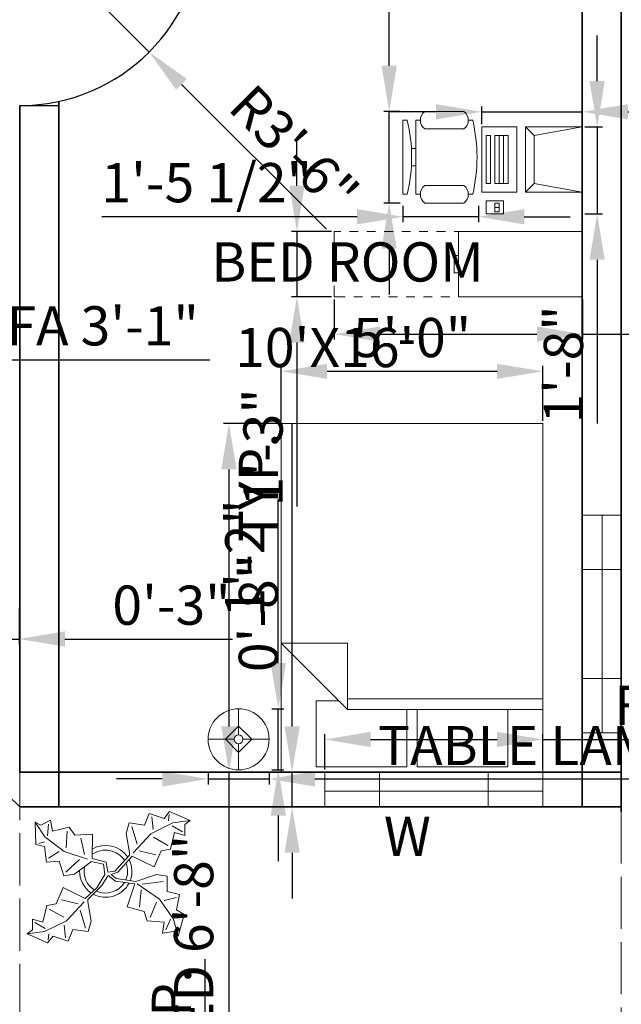
# Model space of a CAD drawing. Units: inches. Extents: x 1956 to 4770, y 1551 to 2596.
# Tile 4 of 10: x 2363 to 2501, y 1865 to 2091. Entities that reach past the tile are written whole.
import ezdxf

# ---------------------------------------------------------------- set-up
doc = ezdxf.new("R2010")
doc.units = ezdxf.units.IN
doc.linetypes.add('ACAD_ISO02W100', pattern=[15, 12, -3])
for name, color, linetype, lineweight in [('A-ANNO-DIMS', 2, 'Continuous', 18), ('A-ANNO-TEXT', 7, 'Continuous', 18), ('A-AREA-IDEN', 7, 'Continuous', 18), ('A-DOOR', 3, 'Continuous', 25), ('A-EQPM', 9, 'Continuous', 18), ('A-FLOR-OVHD', 8, 'ACAD_ISO02W100', 18), ('A-FURN', 8, 'Continuous', 18), ('A-GLAZ', 4, 'Continuous', 18), ('A-WALL', 7, 'Continuous', 35), ('L-PLNT', 116, 'Continuous', 18)]:
    doc.layers.add(name, color=color, linetype=linetype, lineweight=lineweight)
doc.styles.get("Standard").update_dxf_attribs({"font": 'arial.ttf'})
doc.dimstyles.new('ISO-25', dxfattribs={"dimtxt": 9, "dimasz": 10.5, "dimexe": 1.25, "dimexo": 0.625, "dimgap": 2, "dimtad": 1, "dimdec": 1, "dimlunit": 4, "dimtxsty": 'Standard', "dimcen": 2.5, "dimadec": 0, "dimazin": 0, "dimtfac": 1, "dimtdec": 1, "dimtmove": 0, "dimatfit": 3, "dimfxl": 1, "dimarcsym": 0})

# ---------------------------------------------------------------- blocks, each defined once
blk = doc.blocks.new('*D1')
at = {"layer": 'A-ANNO-DIMS', "color": 0, "lineweight": -2, "transparency": 16777216}
for p, q in [((2501.88, 2309.09), (2599.11, 2309.09)), ((2597.86, 2298.59), (2597.86, 1767.59)), ((2501.88, 1757.09), (2599.11, 1757.09))]:
    blk.add_line(p, q, dxfattribs=at)
at = {"layer": 'A-ANNO-DIMS', "color": 0, "transparency": 16777216}
for points in [[(2596.11, 2298.59), (2599.61, 2298.59), (2597.86, 2309.09)], [(2596.11, 1767.59), (2599.61, 1767.59), (2597.86, 1757.09)]]:
    blk.add_solid(points, dxfattribs=at)
at = {"layer": 'Defpoints', "color": 0, "transparency": 16777216}
for p in [(2501.25, 2309.09), (2501.25, 1757.09), (2597.86, 1757.09)]:
    blk.add_point(p, dxfattribs=at)
at = {"layer": 'A-ANNO-DIMS', "color": 0, "transparency": 16777216, "insert": (2591.27, 2033.09), "char_height": 9, "attachment_point": 5, "rotation": 90}
blk.add_mtext("46'", dxfattribs=at)
blk = doc.blocks.new('Bed - Queen')
for p, q in [((0, -80.00003), (0, 0)), ((0, 0), (59.99999, 0)), ((59.99999, 0), (59.99999, -80.00003)), ((7.99999, -1.2), (28.79998, -1.2)), ((7.99999, -14.4), (7.99999, -1.2)), ((28.79998, -1.2), (28.79998, -14.4)), ((31.19999, -1.2), (51.99999, -1.2)), ((31.19999, -14.4), (31.19999, -1.2)), ((51.99999, -1.2), (51.99999, -16.4)), ((0, -14.4), (44.8, -14.4)), ((59.99999, -29.6), (44.8, -14.4)), ((44.8, -14.4), (44.8, -29.6)), ((44.8, -16.8), (0, -16.8)), ((51.99999, -16.4), (46.79936, -16.4)), ((44.8, -29.6), (59.99999, -29.6)), ((59.99999, -80.00003), (0, -80.00003))]:
    blk.add_line(p, q)
blk = doc.blocks.new('Lamp - Table')
for p, q in [((0, 7), (0, 1)), ((0, 3), (-3, 0)), ((3, 0), (0, 3)), ((-1, 0), (-7, 0)), ((-3, 0), (0, -3)), ((0, -3), (3, 0)), ((1, 0), (7, 0)), ((0, -1), (0, -7))]:
    blk.add_line(p, q)
for radius in [7, 1]:
    blk.add_circle((0, 0), radius)
blk = doc.blocks.new('Computer Terminal')
for p, q in [((-10, 11.5), (5, 11.5)), ((-8, 0.5), (-10, 11.5)), ((-10, -1.5), (-10, 11.5)), ((5, 11.5), (3, 0.5)), ((5, 11.5), (5, -1.5)), ((-10, -1.5), (-8, 0.5)), ((3, 0.5), (-8, 0.5)), ((3, 0.5), (5, -1.5)), ((5, -1.5), (-10, -1.5)), ((-10, -11.5), (-10, -3.5)), ((-10, -3.5), (5, -3.5)), ((5, -3.5), (5, -11.5)), ((-8, -5.5), (-8, -8.5)), ((3, -5.5), (-8, -5.5)), ((3, -6.5), (-8, -6.5)), ((3, -8.5), (3, -5.5)), ((10, -6.5), (7, -6.5)), ((7, -6.5), (7, -10.5)), ((10, -10.5), (10, -6.5)), ((-8, -7.5), (3, -7.5)), ((-8, -8.5), (3, -8.5)), ((9.5, -7.5), (7.5, -7.5)), ((7.5, -7.5), (7.5, -8.5)), ((7.5, -8.5), (9.5, -8.5)), ((8.5, -7.5), (8.5, -8.5)), ((9.5, -8.5), (9.5, -7.5)), ((-8, -9.5), (-8, -10.5)), ((3, -9.5), (-8, -9.5)), ((-8, -10.5), (3, -10.5)), ((3, -10.5), (3, -9.5)), ((7, -10.5), (10, -10.5)), ((5, -11.5), (-10, -11.5))]:
    blk.add_line(p, q)
blk = doc.blocks.new('File Cabinet - Letter')
for p, q in [((0, 0), (15, 0)), ((0, -28.5), (0, 0)), ((15, 0), (15, -28.5)), ((15, -28.5), (0, -28.5)), ((0, -29.5), (0, -28.5)), ((5.5, -28.5), (5.5, -29.5)), ((9.5, -29.5), (9.5, -28.5)), ((0, -33.5), (0, -31.5)), ((5.5, -29.5), (9.5, -29.5)), ((15, -30.5), (15, -32.5)), ((0, -37.5), (0, -35.5)), ((15, -34.5), (15, -36.5)), ((0, -41.5), (0, -39.5)), ((15, -38.5), (15, -40.5)), ((15, -42.5), (15, -44.5)), ((0, -45.5), (0, -43.5)), ((15, -46.5), (15, -48.5)), ((0, -49.5), (0, -47.5)), ((0, -53.5), (0, -51.5)), ((15, -50.5), (15, -52.5)), ((0, -57), (0, -55.5)), ((15, -54.5), (15, -57)), ((2.5, -57), (0, -57)), ((6.5, -57), (4.5, -57)), ((10.5, -57), (8.5, -57)), ((15, -57), (12.5, -57))]:
    blk.add_line(p, q)
blk = doc.blocks.new('Chair - Desk')
for p, q in [((-8.5, 0), (-8.5, -1)), ((-8.5, 0), (8.5, 0)), ((8.5, 0), (8.5, -1)), ((-2, -3), (-2, -1.9355)), ((2, -1.9576), (2, -3)), ((-8.5, -3), (-8.5, -4)), ((-8.5, -3), (8.5, -3)), ((8.5, -3), (8.5, -4)), ((-10.5, -5), (-10.5, -14)), ((-6.5, -14), (-6.5, -5)), ((6.5, -5), (6.5, -14)), ((10.5, -14), (10.5, -5)), ((-8.5, -15), (-8.5, -16)), ((8.5, -15), (8.5, -16))]:
    blk.add_line(p, q)
for centre, radius, start, end in [((0, 34.625), 36.625, 256.5803, 283.4197), ((-8.5, -6.5), 2.5, 36.8699, 143.1301), ((8.5, -6.5), 2.5, 36.8699, 143.1301), ((-8.5, -12.5), 2.5, 216.8699, 323.1301), ((8.5, -12.5), 2.5, 216.8699, 323.1301), ((0, 19.625), 36.625, 256.5803, 283.4197)]:
    blk.add_arc(centre, radius, start, end)
blk = doc.blocks.new('Plant - Rubber or Philodendron')
for p, q in [((13.3837, 12.301), (14.68, 13.9039)), ((14.68, 13.9039), (19.3848, 11.8146)), ((-16.2005, 11.4774), (-13.9899, 8.1064)), ((-16.2005, 11.4774), (-14.8639, 10.7964)), ((-16.0159, 6.3329), (-16.2005, 11.4774)), ((-14.8639, 10.7964), (-12.6195, 11.8975)), ((-12.6195, 11.8975), (-12.1909, 9.4345)), ((8.8871, 10.7908), (9.9809, 13.4933)), ((9.9809, 13.4933), (13.3837, 12.301)), ((15.3859, 11.3055), (10.3916, 8.7942)), ((10.5828, 12.6946), (10.8893, 9.7953)), ((14.5816, 13.2037), (14.3848, 11.8033)), ((19.3848, 11.8146), (15.3859, 11.3055)), ((19.3848, 11.8146), (18.1868, 10.9119)), ((-13.3174, 8.325), (-13.0735, 11.0065)), ((-12.1909, 9.4345), (-8.3829, 10.3)), ((-8.8369, 9.409), (-9.0894, 5.6095)), ((-8.3829, 10.3), (-7.0549, 8.501)), ((4.6914, 8.8812), (5.3859, 11.2828)), ((5.3859, 11.2828), (8.8871, 10.7908)), ((5.9878, 10.4842), (7.1971, 6.3869)), ((15.7909, 9.1065), (14.8995, 5.3044)), ((15.2875, 10.6053), (17.5907, 9.2105)), ((18.1925, 8.4119), (15.7909, 9.1065)), ((18.1868, 10.9119), (18.1925, 8.4119)), ((-15.3434, 6.5514), (-13.9984, 6.9884)), ((-13.9899, 8.1064), (-9.5434, 4.7185)), ((-7.0549, 8.501), (-3.0284, 8.6941)), ((-4.8529, 4.012), (-5.7184, 7.82)), ((-3.0284, 8.6941), (-3.0709, 3.1041)), ((4.6914, 8.8812), (5.5014, 4.4831)), ((10.3916, 8.7942), (6.2847, 4.4028)), ((14.2977, 6.1031), (10.9934, 7.9956)), ((-14.0069, 5.8704), (-16.0159, 6.3329)), ((-13.5868, 2.2894), (-14.0069, 5.8704)), ((-13.1329, 3.1804), (-10.6614, 4.727)), ((-9.5434, 4.7185), (-4.1917, 2.9888)), ((7.7005, 4.8881), (11.5025, 3.9967)), ((12.7005, 4.8994), (11.1089, 1.1958)), ((14.8995, 5.3044), (12.7005, 4.8994)), ((-10.6784, 2.491), (-13.5868, 2.2894)), ((-9.5858, -0.8715), (-10.6784, 2.491)), ((-9.1318, 0.0195), (-5.9793, 2.9025)), ((-3.5248, 2.2131), (-3.3011, 2.4355)), ((-3.3011, 2.4355), (-0.5306, 1.7947)), ((-3.0709, 3.1041), (0.0797, 2.3163)), ((0.0797, 2.3163), (0.4866, -0.031)), ((2.1141, 0.2298), (5.4346, 3.9146)), ((6.1032, 3.6844), (2.8262, -0.031)), ((5.4346, 3.9146), (5.5014, 4.4831)), ((11.1089, 1.1958), (6.1032, 3.6844)), ((-7.1228, -0.443), (-3.5248, 2.2131)), ((-0.5306, 1.7947), (-0.2255, -0.5527)), ((-0.5306, 1.7947), (-0.5306, 1.7947)), ((0.4866, -0.031), (2.1141, 0.2298)), ((-7.1228, -0.443), (-9.5858, -0.8715)), ((-2.019, -3.6148), (-0.2255, -0.5527)), ((-0.9375, -3.1608), (0.5883, -0.8135)), ((0.5883, -0.8135), (2.2447, -2.0916)), ((2.8262, -0.031), (1.3003, -0.5527)), ((1.3003, -0.5527), (2.4193, -1.4655)), ((2.2447, -2.0916), (6.7108, -2.6626)), ((2.4193, -1.4655), (6.895, -2.1175)), ((11.6605, -0.5413), (6.895, -2.1175)), ((8.3544, -2.7453), (13.1973, -2.1704)), ((11.6605, -0.5413), (14.1354, -0.8948)), ((14.1354, -0.8948), (14.1354, -4.4304)), ((-11.3237, -7.2629), (-9.7321, -3.5593)), ((-9.7321, -3.5593), (-4.7264, -6.0479)), ((-2.019, -3.6148), (-4.7264, -6.0479)), ((-4.0579, -6.2781), (-0.9375, -3.1608)), ((4.943, -7.9659), (6.7108, -2.6626)), ((12.3677, -6.1981), (7.219, -2.6772)), ((8.125, -4.0768), (7.7715, -7.9659)), ((14.1354, -4.4304), (16.9638, -5.1375)), ((-6.3237, -7.2516), (-10.1257, -6.3602)), ((-4.1246, -6.8466), (-4.0579, -6.2781)), ((15.5496, -10.7943), (12.3677, -6.1981)), ((16.2567, -5.8446), (13.4283, -6.5517)), ((16.9638, -5.1375), (16.2567, -8.673)), ((-14.4141, -11.4699), (-13.5228, -7.6679)), ((-13.5228, -7.6679), (-11.3237, -7.2629)), ((-12.921, -8.4665), (-9.6166, -10.359)), ((-9.0148, -11.1577), (-4.9047, -6.8122)), ((-4.611, -12.8477), (-5.8203, -8.7504)), ((-3.3146, -11.2447), (-4.1246, -6.8466)), ((8.8321, -9.0266), (4.943, -7.9659)), ((9.5392, -11.1479), (8.8321, -9.0266)), ((10.2463, -10.4408), (11.6605, -6.9053)), ((16.2567, -8.673), (18.0245, -9.7337)), ((-16.8157, -10.7754), (-14.4141, -11.4699)), ((-16.8101, -13.2754), (-16.8157, -10.7754)), ((-14.0091, -13.669), (-9.0148, -11.1577)), ((-3.3146, -11.2447), (-4.0092, -13.6463)), ((13.4283, -11.5015), (9.5392, -11.1479)), ((14.8425, -10.7943), (13.7819, -13.2692)), ((16.6103, -14.6834), (15.5496, -10.7943)), ((17.3174, -9.7337), (15.9032, -9.7337)), ((18.0245, -9.7337), (16.6103, -14.6834)), ((-18.008, -14.1781), (-16.8101, -13.2754)), ((-13.9107, -12.9688), (-16.2139, -11.574)), ((-9.206, -15.0581), (-9.5126, -12.1588)), ((-7.5103, -13.1543), (-8.6042, -15.8568)), ((-4.0092, -13.6463), (-7.5103, -13.1543)), ((13.0748, -13.9763), (13.4283, -11.5015)), ((-18.008, -14.1781), (-14.0091, -13.669)), ((-13.3032, -16.2674), (-18.008, -14.1781)), ((-12.0069, -14.6645), (-13.3032, -16.2674)), ((-13.2048, -15.5672), (-13.008, -14.1668)), ((-8.6042, -15.8568), (-12.0069, -14.6645)), ((15.5496, -13.6228), (13.0748, -13.9763)), ((16.6103, -14.6834), (15.5496, -13.6228))]:
    blk.add_line(p, q)
for centre, radius, start, end in [((0, 0), 6.1275, 34.37569, 120.1028), ((-0.0601, -0.2075), 5.2461, 33.82192, 124.9414), ((-0.098, 0.1364), 6.1288, 341.2017, 26.09184), ((0.0308, 0.1664), 6, 178.6147, 235.1169), ((0.0308, 0.1664), 5, 168.1647, 238.6725), ((-0.2664, 0.1682), 5.2775, 338.4094, 20.03007), ((-0.0234, 0.3825), 6.1492, 242.5812, 331.2714), ((-0.1102, 0.4886), 5.2883, 247.3711, 327.472)]:
    blk.add_arc(centre, radius, start, end)
blk = doc.blocks.new('WIN-50IN-WALL9')
for p, q in [((0, 50), (9, 50)), ((4.6, 50), (4.6, 0)), ((0, 37.5), (9, 37.5)), ((9, 12.5), (0, 12.5)), ((9, 0), (1, 0)), ((0, 0), (9, 0))]:
    blk.add_line(p, q)
blk = doc.blocks.new('WIN-50IN-WALL8')
for p, q in [((0, 0), (0, 8)), ((12.5, 0), (12.5, 8)), ((37.5, 8), (37.5, 0)), ((50, 8), (50, 0)), ((0, 3.6), (50, 3.6))]:
    blk.add_line(p, q)
blk = doc.blocks.new('*D29')
at = {"layer": 'A-ANNO-DIMS', "color": 0, "lineweight": -2, "transparency": 16777216}
for p, q in [((2433.25, 1918.71), (2433.25, 1926.84)), ((2483.25, 1918.71), (2483.25, 1926.84)), ((2443.75, 1925.59), (2472.75, 1925.59)), ((2483.25, 1925.59), (2657.56, 1925.59))]:
    blk.add_line(p, q, dxfattribs=at)
at = {"layer": 'A-ANNO-DIMS', "color": 0, "transparency": 16777216}
for points in [[(2443.75, 1927.34), (2443.75, 1923.84), (2433.25, 1925.59)], [(2472.75, 1927.34), (2472.75, 1923.84), (2483.25, 1925.59)]]:
    blk.add_solid(points, dxfattribs=at)
at = {"layer": 'Defpoints', "color": 0, "transparency": 16777216}
for p in [(2483.25, 1925.59), (2433.25, 1918.09), (2483.25, 1918.09)]:
    blk.add_point(p, dxfattribs=at)
at = {"layer": 'A-ANNO-DIMS', "color": 0, "transparency": 16777216, "insert": (2575.65, 1932.24), "char_height": 9, "attachment_point": 5}
blk.add_mtext('FRONT WINDOW 4\'-2" TYP.', dxfattribs=at)
blk = doc.blocks.new('*D30')
at = {"layer": 'A-ANNO-DIMS', "color": 0, "lineweight": -2, "transparency": 16777216}
for p, q in [((2425.75, 1928.59), (2425.75, 1997.95)), ((2432.63, 1918.09), (2424.5, 1918.09)), ((2425.75, 1910.09), (2425.75, 1918.09)), ((2432.63, 1910.09), (2424.5, 1910.09)), ((2425.75, 1899.59), (2425.75, 1889.09))]:
    blk.add_line(p, q, dxfattribs=at)
at = {"layer": 'A-ANNO-DIMS', "color": 0, "transparency": 16777216}
for points in [[(2424, 1928.59), (2427.5, 1928.59), (2425.75, 1918.09)], [(2424, 1899.59), (2427.5, 1899.59), (2425.75, 1910.09)]]:
    blk.add_solid(points, dxfattribs=at)
at = {"layer": 'Defpoints', "color": 0, "transparency": 16777216}
for p in [(2425.75, 1918.09), (2433.25, 1918.09), (2433.25, 1910.09)]:
    blk.add_point(p, dxfattribs=at)
at = {"layer": 'A-ANNO-DIMS', "color": 0, "transparency": 16777216, "insert": (2419.16, 1968.52), "char_height": 9, "attachment_point": 5, "rotation": 90}
blk.add_mtext('0\'-8" TYP.', dxfattribs=at)
blk = doc.blocks.new('*D31')
at = {"layer": 'A-ANNO-DIMS', "color": 0, "lineweight": -2, "transparency": 16777216}
for p, q in [((2294, 2017.6), (2294, 2011.46)), ((2330.76, 2017.6), (2330.76, 2011.46)), ((2304.5, 2012.71), (2320.26, 2012.71)), ((2330.76, 2012.71), (2406.87, 2012.71))]:
    blk.add_line(p, q, dxfattribs=at)
at = {"layer": 'A-ANNO-DIMS', "color": 0, "transparency": 16777216}
for points in [[(2304.5, 2014.46), (2304.5, 2010.96), (2294, 2012.71)], [(2320.26, 2014.46), (2320.26, 2010.96), (2330.76, 2012.71)]]:
    blk.add_solid(points, dxfattribs=at)
at = {"layer": 'Defpoints', "color": 0, "transparency": 16777216}
for p in [(2294, 2018.23), (2330.76, 2018.23), (2330.76, 2012.71)]:
    blk.add_point(p, dxfattribs=at)
at = {"layer": 'A-ANNO-DIMS', "color": 0, "transparency": 16777216, "insert": (2374.07, 2019.37), "char_height": 9, "attachment_point": 5}
blk.add_mtext('SOFA 3\'-1"', dxfattribs=at)
blk = doc.blocks.new('*D40')
at = {"layer": 'A-ANNO-DIMS', "color": 0, "lineweight": -2, "transparency": 16777216}
for p, q in [((2405.81, 1805.68), (2405.81, 1875.19)), ((2400.82, 1805.68), (2407.06, 1805.68)), ((2405.81, 1786.01), (2405.81, 1795.18)), ((2400.82, 1775.51), (2407.06, 1775.51))]:
    blk.add_line(p, q, dxfattribs=at)
at = {"layer": 'A-ANNO-DIMS', "color": 0, "transparency": 16777216}
for points in [[(2404.06, 1795.18), (2407.56, 1795.18), (2405.81, 1805.68)], [(2404.06, 1786.01), (2407.56, 1786.01), (2405.81, 1775.51)]]:
    blk.add_solid(points, dxfattribs=at)
at = {"layer": 'Defpoints', "color": 0, "transparency": 16777216}
for p in [(2400.2, 1805.68), (2405.81, 1805.68), (2400.2, 1775.51)]:
    blk.add_point(p, dxfattribs=at)
at = {"layer": 'A-ANNO-DIMS', "color": 0, "transparency": 16777216, "insert": (2399.21, 1845.69), "char_height": 9, "attachment_point": 5, "rotation": 90}
blk.add_mtext('2\'-6" TYP.', dxfattribs=at)
blk = doc.blocks.new('*D45')
at = {"layer": 'A-ANNO-DIMS', "color": 0, "lineweight": -2, "transparency": 16777216}
for p, q in [((2422.63, 1998.09), (2410, 1998.09)), ((2411.25, 1987.59), (2411.25, 1928.59)), ((2422.63, 1918.09), (2410, 1918.09)), ((2411.25, 1918.09), (2411.25, 1802.13))]:
    blk.add_line(p, q, dxfattribs=at)
at = {"layer": 'A-ANNO-DIMS', "color": 0, "transparency": 16777216}
for points in [[(2409.5, 1987.59), (2413, 1987.59), (2411.25, 1998.09)], [(2409.5, 1928.59), (2413, 1928.59), (2411.25, 1918.09)]]:
    blk.add_solid(points, dxfattribs=at)
at = {"layer": 'Defpoints', "color": 0, "transparency": 16777216}
for p in [(2423.25, 1998.09), (2411.25, 1918.09), (2423.25, 1918.09)]:
    blk.add_point(p, dxfattribs=at)
at = {"layer": 'A-ANNO-DIMS', "color": 0, "transparency": 16777216, "insert": (2404.32, 1854.86), "char_height": 9, "attachment_point": 5, "rotation": 90}
blk.add_mtext('QUEEN BED 6\'-8"', dxfattribs=at)
blk = doc.blocks.new('*D46')
at = {"layer": 'A-ANNO-DIMS', "color": 0, "lineweight": -2, "transparency": 16777216}
for p, q in [((2423.25, 1998.71), (2423.25, 2011.34)), ((2472.75, 2010.09), (2433.75, 2010.09)), ((2483.25, 1998.71), (2483.25, 2011.34))]:
    blk.add_line(p, q, dxfattribs=at)
at = {"layer": 'A-ANNO-DIMS', "color": 0, "transparency": 16777216}
for points in [[(2433.75, 2011.84), (2433.75, 2008.34), (2423.25, 2010.09)], [(2472.75, 2011.84), (2472.75, 2008.34), (2483.25, 2010.09)]]:
    blk.add_solid(points, dxfattribs=at)
at = {"layer": 'Defpoints', "color": 0, "transparency": 16777216}
for p in [(2423.25, 2010.09), (2423.25, 1998.09), (2483.25, 1998.09)]:
    blk.add_point(p, dxfattribs=at)
at = {"layer": 'A-ANNO-DIMS', "color": 0, "transparency": 16777216, "insert": (2453.25, 2016.68), "char_height": 9, "attachment_point": 5}
blk.add_mtext('5\'-0"', dxfattribs=at)
blk = doc.blocks.new('*D47')
at = {"layer": 'A-ANNO-DIMS', "color": 0, "lineweight": -2, "transparency": 16777216}
for p, q in [((2406.47, 1918), (2406.47, 1915.27)), ((2420.47, 1918), (2420.47, 1915.27)), ((2395.97, 1916.52), (2385.47, 1916.52)), ((2406.47, 1916.52), (2420.47, 1916.52)), ((2430.97, 1916.52), (2550.67, 1916.52))]:
    blk.add_line(p, q, dxfattribs=at)
at = {"layer": 'A-ANNO-DIMS', "color": 0, "transparency": 16777216}
for points in [[(2395.97, 1918.27), (2395.97, 1914.77), (2406.47, 1916.52)], [(2430.97, 1918.27), (2430.97, 1914.77), (2420.47, 1916.52)]]:
    blk.add_solid(points, dxfattribs=at)
at = {"layer": 'Defpoints', "color": 0, "transparency": 16777216}
for p in [(2406.47, 1918.62), (2420.47, 1918.62), (2420.47, 1916.52)]:
    blk.add_point(p, dxfattribs=at)
at = {"layer": 'A-ANNO-DIMS', "color": 0, "transparency": 16777216, "insert": (2496.07, 1923.04), "char_height": 9, "attachment_point": 5}
blk.add_mtext('TABLE LAMP 1\'-2"', dxfattribs=at)
blk = doc.blocks.new('*D48')
at = {"layer": 'A-ANNO-DIMS', "color": 0, "lineweight": -2, "transparency": 16777216}
for p, q in [((2422.57, 1943.12), (2422.57, 1980.7)), ((2421.09, 1932.62), (2423.82, 1932.62)), ((2422.57, 1918.62), (2422.57, 1932.62)), ((2421.09, 1918.62), (2423.82, 1918.62)), ((2422.57, 1908.12), (2422.57, 1897.62))]:
    blk.add_line(p, q, dxfattribs=at)
at = {"layer": 'A-ANNO-DIMS', "color": 0, "transparency": 16777216}
for points in [[(2420.82, 1943.12), (2424.32, 1943.12), (2422.57, 1932.62)], [(2420.82, 1908.12), (2424.32, 1908.12), (2422.57, 1918.62)]]:
    blk.add_solid(points, dxfattribs=at)
at = {"layer": 'Defpoints', "color": 0, "transparency": 16777216}
for p in [(2420.47, 1932.62), (2422.57, 1932.62), (2420.47, 1918.62)]:
    blk.add_point(p, dxfattribs=at)
at = {"layer": 'A-ANNO-DIMS', "color": 0, "transparency": 16777216, "insert": (2416.05, 1967.16), "char_height": 9, "attachment_point": 5, "rotation": 90}
blk.add_mtext('1\'-2"', dxfattribs=at)
blk = doc.blocks.new('*D53')
at = {"layer": 'A-ANNO-DIMS', "color": 0, "lineweight": -2, "transparency": 16777216}
for p, q in [((2469.27, 2066.83), (2469.27, 2070.91)), ((2492.27, 2066.83), (2492.27, 2070.91)), ((2458.77, 2069.66), (2448.27, 2069.66)), ((2469.27, 2069.66), (2492.27, 2069.66)), ((2502.77, 2069.66), (2623.52, 2069.66))]:
    blk.add_line(p, q, dxfattribs=at)
at = {"layer": 'A-ANNO-DIMS', "color": 0, "transparency": 16777216}
for points in [[(2458.77, 2071.41), (2458.77, 2067.91), (2469.27, 2069.66)], [(2502.77, 2071.41), (2502.77, 2067.91), (2492.27, 2069.66)]]:
    blk.add_solid(points, dxfattribs=at)
at = {"layer": 'Defpoints', "color": 0, "transparency": 16777216}
for p in [(2492.27, 2069.66), (2469.27, 2066.21), (2492.27, 2066.21)]:
    blk.add_point(p, dxfattribs=at)
at = {"layer": 'A-ANNO-DIMS', "color": 0, "transparency": 16777216, "insert": (2568.4, 2076.31), "char_height": 9, "attachment_point": 5}
blk.add_mtext('COMPUTER 1\'-11"', dxfattribs=at)
blk = doc.blocks.new('*D54')
at = {"layer": 'A-ANNO-DIMS', "color": 0, "lineweight": -2, "transparency": 16777216}
for p, q in [((2495.72, 2076.71), (2495.72, 2087.21)), ((2492.9, 2066.21), (2496.97, 2066.21)), ((2495.72, 2066.21), (2495.72, 2046.21)), ((2492.9, 2046.21), (2496.97, 2046.21)), ((2495.72, 2035.71), (2495.72, 1998.13))]:
    blk.add_line(p, q, dxfattribs=at)
at = {"layer": 'A-ANNO-DIMS', "color": 0, "transparency": 16777216}
for points in [[(2493.97, 2076.71), (2497.47, 2076.71), (2495.72, 2066.21)], [(2493.97, 2035.71), (2497.47, 2035.71), (2495.72, 2046.21)]]:
    blk.add_solid(points, dxfattribs=at)
at = {"layer": 'Defpoints', "color": 0, "transparency": 16777216}
for p in [(2492.27, 2066.21), (2492.27, 2046.21), (2495.72, 2046.21)]:
    blk.add_point(p, dxfattribs=at)
at = {"layer": 'A-ANNO-DIMS', "color": 0, "transparency": 16777216, "insert": (2489.13, 2011.67), "char_height": 9, "attachment_point": 5, "rotation": 90}
blk.add_mtext('1\'-8"', dxfattribs=at)
blk = doc.blocks.new('*D55')
at = {"layer": 'A-ANNO-DIMS', "color": 0, "lineweight": -2, "transparency": 16777216}
for p, q in [((2435.39, 2026.56), (2435.39, 2017.38)), ((2492.39, 2026.56), (2492.39, 2017.38)), ((2445.89, 2018.63), (2481.89, 2018.63)), ((2492.39, 2018.63), (2618.34, 2018.63))]:
    blk.add_line(p, q, dxfattribs=at)
at = {"layer": 'A-ANNO-DIMS', "color": 0, "transparency": 16777216}
for points in [[(2445.89, 2020.38), (2445.89, 2016.88), (2435.39, 2018.63)], [(2481.89, 2020.38), (2481.89, 2016.88), (2492.39, 2018.63)]]:
    blk.add_solid(points, dxfattribs=at)
at = {"layer": 'Defpoints', "color": 0, "transparency": 16777216}
for p in [(2435.39, 2027.18), (2492.39, 2027.18), (2492.39, 2018.63)]:
    blk.add_point(p, dxfattribs=at)
at = {"layer": 'A-ANNO-DIMS', "color": 0, "transparency": 16777216, "insert": (2560.61, 2025.28), "char_height": 9, "attachment_point": 5}
blk.add_mtext('FILE CABINET 4\'-9"', dxfattribs=at)
blk = doc.blocks.new('*D56')
at = {"layer": 'A-ANNO-DIMS', "color": 0, "lineweight": -2, "transparency": 16777216}
for p, q in [((2426.84, 2052.68), (2426.84, 2063.18)), ((2434.77, 2042.18), (2425.59, 2042.18)), ((2426.84, 2042.18), (2426.84, 2027.18)), ((2434.77, 2027.18), (2425.59, 2027.18)), ((2426.84, 2016.68), (2426.84, 1979.1))]:
    blk.add_line(p, q, dxfattribs=at)
at = {"layer": 'A-ANNO-DIMS', "color": 0, "transparency": 16777216}
for points in [[(2425.09, 2052.68), (2428.59, 2052.68), (2426.84, 2042.18)], [(2425.09, 2016.68), (2428.59, 2016.68), (2426.84, 2027.18)]]:
    blk.add_solid(points, dxfattribs=at)
at = {"layer": 'Defpoints', "color": 0, "transparency": 16777216}
for p in [(2435.39, 2042.18), (2426.84, 2027.18), (2435.39, 2027.18)]:
    blk.add_point(p, dxfattribs=at)
at = {"layer": 'A-ANNO-DIMS', "color": 0, "transparency": 16777216, "insert": (2420.24, 1992.64), "char_height": 9, "attachment_point": 5, "rotation": 90}
blk.add_mtext('1\'-3"', dxfattribs=at)
blk = doc.blocks.new('*D57')
at = {"layer": 'A-ANNO-DIMS', "color": 0, "lineweight": -2, "transparency": 16777216}
for p, q in [((2448.01, 2080.23), (2448.01, 2198.55)), ((2450.54, 2069.73), (2446.76, 2069.73)), ((2448.01, 2048.73), (2448.01, 2069.73)), ((2450.54, 2048.73), (2446.76, 2048.73)), ((2448.01, 2038.23), (2448.01, 2027.73))]:
    blk.add_line(p, q, dxfattribs=at)
at = {"layer": 'A-ANNO-DIMS', "color": 0, "transparency": 16777216}
for points in [[(2446.26, 2080.23), (2449.76, 2080.23), (2448.01, 2069.73)], [(2446.26, 2038.23), (2449.76, 2038.23), (2448.01, 2048.73)]]:
    blk.add_solid(points, dxfattribs=at)
at = {"layer": 'Defpoints', "color": 0, "transparency": 16777216}
for p in [(2448.01, 2069.73), (2451.16, 2069.73), (2451.16, 2048.73)]:
    blk.add_point(p, dxfattribs=at)
at = {"layer": 'A-ANNO-DIMS', "color": 0, "transparency": 16777216, "insert": (2441.36, 2144.64), "char_height": 9, "attachment_point": 5, "rotation": 90}
blk.add_mtext('DESK CHAIR 1\'-9"', dxfattribs=at)
blk = doc.blocks.new('*D58')
at = {"layer": 'A-ANNO-DIMS', "color": 0, "lineweight": -2, "transparency": 16777216}
for p, q in [((2451.16, 2048.1), (2451.16, 2044.33)), ((2468.49, 2048.1), (2468.49, 2044.33)), ((2440.66, 2045.58), (2382.11, 2045.58)), ((2468.49, 2045.58), (2451.16, 2045.58)), ((2478.99, 2045.58), (2489.49, 2045.58))]:
    blk.add_line(p, q, dxfattribs=at)
at = {"layer": 'A-ANNO-DIMS', "color": 0, "transparency": 16777216}
for points in [[(2440.66, 2047.33), (2440.66, 2043.83), (2451.16, 2045.58)], [(2478.99, 2047.33), (2478.99, 2043.83), (2468.49, 2045.58)]]:
    blk.add_solid(points, dxfattribs=at)
at = {"layer": 'Defpoints', "color": 0, "transparency": 16777216}
for p in [(2451.16, 2048.73), (2468.49, 2048.73), (2451.16, 2045.58)]:
    blk.add_point(p, dxfattribs=at)
at = {"layer": 'A-ANNO-DIMS', "color": 0, "transparency": 16777216, "insert": (2406.14, 2052.23), "char_height": 9, "attachment_point": 5}
blk.add_mtext('1\'-5 1/2"', dxfattribs=at)
blk = doc.blocks.new('*D61')
at = {"layer": 'A-ANNO-DIMS', "color": 0, "lineweight": -2, "transparency": 16777216}
for p, q in [((2359.65, 2008.45), (2351.23, 2008.45)), ((2352.48, 1997.95), (2352.48, 1966.95)), ((2359.65, 1956.45), (2351.23, 1956.45)), ((2352.48, 1956.45), (2352.48, 1842.3))]:
    blk.add_line(p, q, dxfattribs=at)
at = {"layer": 'A-ANNO-DIMS', "color": 0, "transparency": 16777216}
for points in [[(2350.73, 1997.95), (2354.23, 1997.95), (2352.48, 2008.45)], [(2350.73, 1966.95), (2354.23, 1966.95), (2352.48, 1956.45)]]:
    blk.add_solid(points, dxfattribs=at)
at = {"layer": 'Defpoints', "color": 0, "transparency": 16777216}
for p in [(2360.28, 2008.45), (2352.48, 1956.45), (2360.28, 1956.45)]:
    blk.add_point(p, dxfattribs=at)
at = {"layer": 'A-ANNO-DIMS', "color": 0, "transparency": 16777216, "insert": (2345.9, 1894.13), "char_height": 9, "attachment_point": 5, "rotation": 90}
blk.add_mtext('MEDIA UNIT 4\'-4"', dxfattribs=at)
blk = doc.blocks.new('*D62')
at = {"layer": 'A-ANNO-DIMS', "color": 0, "lineweight": -2, "transparency": 16777216}
for p, q in [((2360.28, 1955.83), (2360.28, 1947.4)), ((2363.11, 1955.83), (2363.11, 1947.4)), ((2349.78, 1948.65), (2339.28, 1948.65)), ((2360.28, 1948.65), (2363.11, 1948.65)), ((2373.61, 1948.65), (2412.03, 1948.65))]:
    blk.add_line(p, q, dxfattribs=at)
at = {"layer": 'A-ANNO-DIMS', "color": 0, "transparency": 16777216}
for points in [[(2349.78, 1950.4), (2349.78, 1946.9), (2360.28, 1948.65)], [(2373.61, 1950.4), (2373.61, 1946.9), (2363.11, 1948.65)]]:
    blk.add_solid(points, dxfattribs=at)
at = {"layer": 'Defpoints', "color": 0, "transparency": 16777216}
for p in [(2360.28, 1956.45), (2363.11, 1956.45), (2363.11, 1948.65)]:
    blk.add_point(p, dxfattribs=at)
at = {"layer": 'A-ANNO-DIMS', "color": 0, "transparency": 16777216, "insert": (2398.07, 1955.25), "char_height": 9, "attachment_point": 5}
blk.add_mtext('0\'-3"', dxfattribs=at)
blk = doc.blocks.new('*D104')
at = {"layer": 'A-ANNO-DIMS', "color": 0, "lineweight": -2, "transparency": 16777216}
for p, q in [((2291.19, 1978.77), (2325.25, 1946.33)), ((2363.3, 1910.09), (2332.85, 1939.09))]:
    blk.add_line(p, q, dxfattribs=at)
at = {"layer": 'A-ANNO-DIMS', "color": 0, "transparency": 16777216}
blk.add_solid([(2326.46, 1947.59), (2324.04, 1945.06), (2332.85, 1939.09)], dxfattribs=at)
at = {"layer": 'Defpoints', "color": 0, "transparency": 16777216}
for p in [(2332.85, 1939.09), (2363.3, 1910.09)]:
    blk.add_point(p, dxfattribs=at)
at = {"layer": 'A-ANNO-DIMS', "color": 0, "transparency": 16777216, "insert": (2308.97, 1970.95), "char_height": 9, "attachment_point": 5, "rotation": 316.3978}
blk.add_mtext('R3\'-6"', dxfattribs=at)
blk = doc.blocks.new('*D105')
at = {"layer": 'A-ANNO-DIMS', "color": 0, "lineweight": -2, "transparency": 16777216}
for p, q in [((2363.25, 2113.09), (2392.95, 2083.39)), ((2433.64, 2042.7), (2400.38, 2075.96))]:
    blk.add_line(p, q, dxfattribs=at)
at = {"layer": 'A-ANNO-DIMS', "color": 0, "transparency": 16777216}
blk.add_solid([(2401.61, 2077.2), (2399.14, 2074.73), (2392.95, 2083.39)], dxfattribs=at)
at = {"layer": 'Defpoints', "color": 0, "transparency": 16777216}
for p in [(2363.25, 2113.09), (2392.95, 2083.39)]:
    blk.add_point(p, dxfattribs=at)
at = {"layer": 'A-ANNO-DIMS', "color": 0, "transparency": 16777216, "insert": (2425.39, 2060.29), "char_height": 9, "attachment_point": 5, "rotation": 315.0003}
blk.add_mtext('R3\'-6"', dxfattribs=at)

msp = doc.modelspace()

# ---------------------------------------------------------------- linework, layer by layer
at = {"layer": 'A-DOOR'}
msp.add_line((2363.25, 2071.09), (2372.25, 2071.09), dxfattribs=at)
msp.add_arc((2363.25, 2113.09), 42, 270, 0, dxfattribs=at)
at = {"layer": 'A-FLOR-OVHD'}
for p, q in [((2363.25, 1802.09), (2363.25, 1918.09)), ((2501.25, 1909.09), (2501.25, 1757.09))]:
    msp.add_line(p, q, dxfattribs=at)
at = {"layer": 'A-GLAZ'}
for p, q in [((2492.25, 1927.09), (2501.25, 1927.09)), ((2483.25, 1918.09), (2483.25, 1910.09))]:
    msp.add_line(p, q, dxfattribs=at)
at = {"layer": 'A-WALL'}
for p, q in [((2501.25, 2309.09), (2501.25, 1909.09)), ((2492.25, 2176.09), (2492.25, 1910.09)), ((2363.25, 1918.09), (2363.25, 2071.09)), ((2372.25, 1918.09), (2372.25, 2072.06)), ((2372.25, 1910.09), (2372.25, 2071.09)), ((2363.25, 1918.09), (2501.25, 1918.09)), ((2501.25, 1910.09), (2363.25, 1910.09))]:
    msp.add_line(p, q, dxfattribs=at)

# ---------------------------------------------------------------- block references
at = {"layer": 'A-EQPM', "rotation": 270}
msp.add_blockref('Computer Terminal', (2480.77, 2056.21), dxfattribs=at)
at = {"layer": 'A-FURN'}
for name, p, rotation in [('Chair - Desk', (2451.16, 2059.23), 90), ('File Cabinet - Letter', (2492.39, 2042.18), 270), ('Bed - Queen', (2483.25, 1918.09), 180)]:
    msp.add_blockref(name, p, dxfattribs=dict(at, rotation=rotation))
msp.add_blockref('Lamp - Table', (2413.47, 1925.62), dxfattribs=at)
at = {"layer": 'A-GLAZ'}
for name, p in [('WIN-50IN-WALL9', (2492.25, 1927.09)), ('WIN-50IN-WALL8', (2433.25, 1910.09))]:
    msp.add_blockref(name, p, dxfattribs=at)
at = {"layer": 'L-PLNT'}
msp.add_blockref('Plant - Rubber or Philodendron', (2382.97, 1895.14), dxfattribs=at)

# ---------------------------------------------------------------- texts
at = {"layer": 'A-ANNO-TEXT'}
msp.add_text('         W ', height=9, dxfattribs=at).set_placement((2422.04, 1898.86))
at = {"layer": 'A-AREA-IDEN'}
for s, p in [('BED ROOM', (2407.18, 2030.7)), ("  10'X16'", (2407.18, 2011.05))]:
    msp.add_text(s, height=9, dxfattribs=at).set_placement(p)

# ---------------------------------------------------------------- dimensions: what is measured, and where the dimension line sits
at = {"layer": 'A-ANNO-DIMS'}
for base, p1, p2, angle, override, picture, middle in [((2597.86, 1757.09), (2501.25, 2309.09), (2501.25, 1757.09), 90, {"dimclrd": 0, "dimclre": 0, "dimclrt": 0}, '*D1', (2591.27, 2033.09)), ((2495.72, 2046.21), (2492.27, 2066.21), (2492.27, 2046.21), 270, {"dimdec": 1, "dimlfac": 1, "dimrnd": 0, "dimzin": 1, "dimdsep": 46, "dimlunit": 4, "dimfrac": 2}, '*D54', (2489.13, 2011.67)), ((2451.16, 2045.58), (2468.49, 2048.73), (2451.16, 2048.73), 180, {"dimdec": 1, "dimlfac": 1, "dimrnd": 0, "dimzin": 1, "dimdsep": 46, "dimlunit": 4, "dimfrac": 2}, '*D58', (2406.14, 2052.23)), ((2426.84, 2027.18), (2435.39, 2042.18), (2435.39, 2027.18), 270, {"dimdec": 1, "dimlfac": 1, "dimrnd": 0, "dimzin": 1, "dimdsep": 46, "dimlunit": 4, "dimfrac": 2}, '*D56', (2420.24, 1992.64)), ((2423.25, 2010.09), (2483.25, 1998.09), (2423.25, 1998.09), 180, {"dimdec": 1, "dimlfac": 1, "dimrnd": 0, "dimzin": 1, "dimdsep": 46, "dimlunit": 4, "dimfrac": 2}, '*D46', (2453.25, 2016.68)), ((2422.57, 1932.62), (2420.47, 1918.62), (2420.47, 1932.62), 90, {"dimdec": 1, "dimlfac": 1, "dimrnd": 0, "dimzin": 1, "dimdsep": 46, "dimlunit": 4, "dimfrac": 2}, '*D48', (2416.05, 1967.16))]:
    dim = msp.add_linear_dim(base=base, p1=p1, p2=p2, angle=angle, dimstyle='ISO-25', override=override, dxfattribs=at)
    dim.commit()
    dim.dimension.update_dxf_attribs({"geometry": picture, "text_midpoint": middle})
for base, p1, p2, angle, text, picture, middle in [((2448.01, 2069.73), (2451.16, 2048.73), (2451.16, 2069.73), 90, 'DESK CHAIR <>', '*D57', (2441.36, 2144.64)), ((2352.48, 1956.45), (2360.28, 2008.45), (2360.28, 1956.45), 270, 'MEDIA UNIT <>', '*D61', (2345.9, 1894.13)), ((2411.25, 1918.09), (2423.25, 1998.09), (2423.25, 1918.09), 270, 'QUEEN BED <>', '*D45', (2404.32, 1854.86)), ((2425.75, 1918.09), (2433.25, 1910.09), (2433.25, 1918.09), 90, '<> TYP.', '*D30', (2419.16, 1968.52)), ((2405.81, 1805.68), (2400.2, 1775.51), (2400.2, 1805.68), 90, '<> TYP.', '*D40', (2399.21, 1845.69))]:
    dim = msp.add_linear_dim(base=base, p1=p1, p2=p2, angle=angle, text=text, dimstyle='ISO-25', override={"dimdec": 1, "dimlfac": 1, "dimrnd": 0, "dimzin": 1, "dimdsep": 46, "dimlunit": 4, "dimfrac": 2}, dxfattribs=at)
    dim.commit()
    dim.dimension.update_dxf_attribs({"geometry": picture, "text_midpoint": middle})
for center, mpoint, picture, middle in [((2363.25, 2113.09), (2392.95, 2083.39), '*D105', (2425.39, 2060.29)), ((2363.30339, 1910.08628), (2332.85306, 1939.08594), '*D104', (2308.96721, 1970.9456))]:
    dim = msp.add_radius_dim(center=center, mpoint=mpoint, dimstyle='ISO-25', override={"dimdec": 1, "dimlfac": 1, "dimrnd": 0, "dimzin": 1, "dimdsep": 46, "dimlunit": 4, "dimfrac": 2}, dxfattribs=at)
    dim.commit()
    dim.dimension.update_dxf_attribs({"geometry": picture, "text_midpoint": middle})
for base, p1, p2, text, picture, middle in [((2492.27, 2069.66), (2469.27, 2066.21), (2492.27, 2066.21), 'COMPUTER <>', '*D53', (2568.4, 2076.31)), ((2492.39, 2018.63), (2435.39, 2027.18), (2492.39, 2027.18), 'FILE CABINET <>', '*D55', (2560.61, 2025.28)), ((2330.76, 2012.71), (2294, 2018.23), (2330.76, 2018.23), 'SOFA <>', '*D31', (2374.07, 2019.37)), ((2483.25, 1925.59), (2433.25, 1918.09), (2483.25, 1918.09), 'FRONT WINDOW <> TYP.', '*D29', (2575.65, 1932.24)), ((2420.47, 1916.52), (2406.47, 1918.62), (2420.47, 1918.62), 'TABLE LAMP <>', '*D47', (2496.07, 1923.04))]:
    dim = msp.add_linear_dim(base=base, p1=p1, p2=p2, text=text, dimstyle='ISO-25', override={"dimdec": 1, "dimlfac": 1, "dimrnd": 0, "dimzin": 1, "dimdsep": 46, "dimlunit": 4, "dimfrac": 2}, dxfattribs=at)
    dim.commit()
    dim.dimension.update_dxf_attribs({"geometry": picture, "text_midpoint": middle})
dim = msp.add_linear_dim(base=(2363.11, 1948.65), p1=(2360.28, 1956.45), p2=(2363.11, 1956.45), dimstyle='ISO-25', override={"dimdec": 1, "dimlfac": 1, "dimrnd": 0, "dimzin": 1, "dimdsep": 46, "dimlunit": 4, "dimfrac": 2}, dxfattribs=at)
dim.commit()
dim.dimension.update_dxf_attribs({"geometry": '*D62', "text_midpoint": (2398.07, 1955.25)})

doc.saveas('drawing.dxf')
